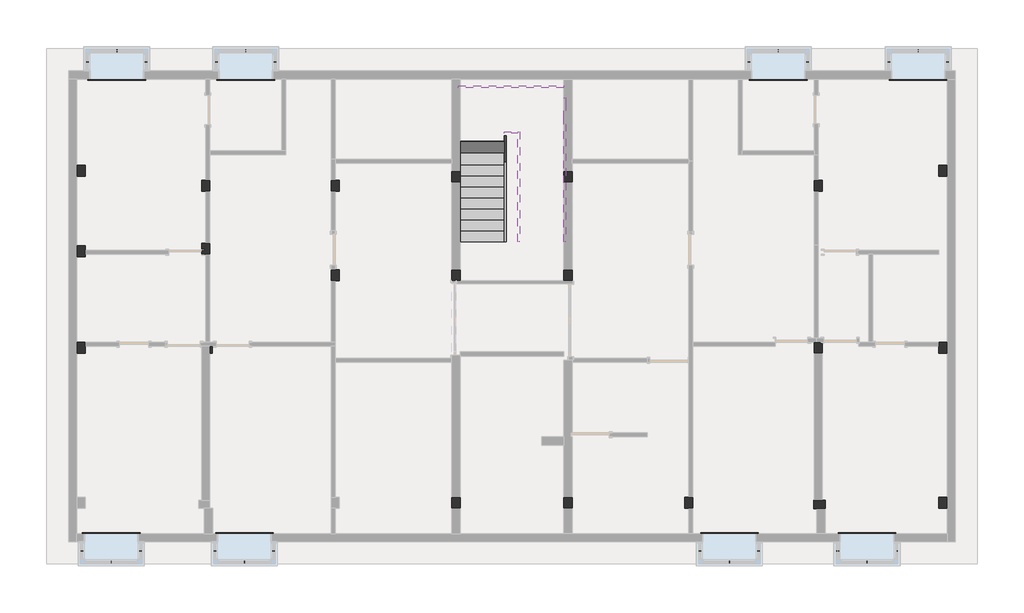
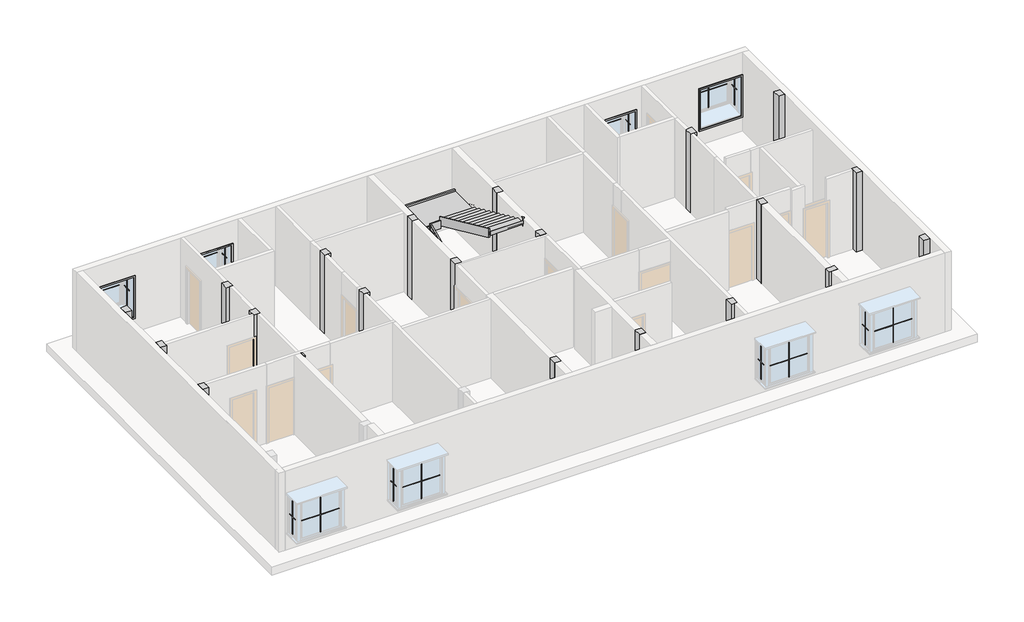
# One storey, part 3 of 3: 32 proxies, 21 columns, 6 members, 1 stair flight.
"""IFC4 building model written with IfcOpenShell, lengths in millimetres."""

from ifc_helpers import new_model, si_unit, frame, origin, place, context, project, spatial, polyline, outline, extrude, faceted_brep, transform, mapped, element, save
from components import m_muntin_pattern_2x2_m_muntin_pattern_2x2_c1fd4460, m_muntin_pattern_2x2_m_muntin_pattern_2x2_777b163a, m_trim_window_interior_flat_picture_frame_44e8afef, stair_flight_5ae6432b

model = new_model("IFC4")

# Units and contexts
model_context = context("Model", 3, world=origin())
ifc_project = project(units=[si_unit("LENGTHUNIT", "METRE", prefix="MILLI")], contexts=[model_context])

# Site, building, storey
site = spatial("IfcSite", under=ifc_project)
building = spatial("IfcBuilding", under=site)
storey = spatial("IfcBuildingStorey", under=building, Elevation=6400.8)

# Proxies
placement = place(None, origin())
m_muntin_pattern_2x2_m_muntin_pattern_2x2_shape = m_muntin_pattern_2x2_m_muntin_pattern_2x2_c1fd4460(model_context)
element("IfcBuildingElementProxy", 1, Name="M_Muntin Pattern_2x2 : M_Muntin Pattern_2x2", ObjectType="M_Muntin Pattern_2x2 : M_Muntin Pattern_2x2", at=placement, inside=storey, context=model_context, shape_type="MappedRepresentation", body=[
    mapped(m_muntin_pattern_2x2_m_muntin_pattern_2x2_shape, transform((-11500.7987957, -5499.9182661, 7121.45), x_axis=(-1.0, 0.0, 0.0), y_axis=(0.0, -1.0, 0.0), z_axis=(0.0, 0.0, 1.0))),
])
element("IfcBuildingElementProxy", 2, Name="M_Muntin Pattern_2x2 : M_Muntin Pattern_2x2", ObjectType="M_Muntin Pattern_2x2 : M_Muntin Pattern_2x2", at=placement, inside=storey, context=model_context, shape_type="MappedRepresentation", body=[
    mapped(m_muntin_pattern_2x2_m_muntin_pattern_2x2_shape, transform((-7819.250543, -5499.9182661, 7121.45), x_axis=(-1.0, 0.0, 0.0), y_axis=(0.0, -1.0, 0.0), z_axis=(0.0, 0.0, 1.0))),
])
element("IfcBuildingElementProxy", 3, Name="M_Muntin Pattern_2x2 : M_Muntin Pattern_2x2", ObjectType="M_Muntin Pattern_2x2 : M_Muntin Pattern_2x2", at=placement, inside=storey, context=model_context, shape_type="MappedRepresentation", body=[
    mapped(m_muntin_pattern_2x2_m_muntin_pattern_2x2_shape, transform((5599.7512082, -5499.9182661, 7121.45), x_axis=(-1.0, 0.0, 0.0), y_axis=(0.0, -1.0, 0.0), z_axis=(0.0, 0.0, 1.0))),
])
element("IfcBuildingElementProxy", 4, Name="M_Muntin Pattern_2x2 : M_Muntin Pattern_2x2", ObjectType="M_Muntin Pattern_2x2 : M_Muntin Pattern_2x2", at=placement, inside=storey, context=model_context, shape_type="MappedRepresentation", body=[
    mapped(m_muntin_pattern_2x2_m_muntin_pattern_2x2_shape, transform((9408.6146942, -5499.9182662, 7121.45), x_axis=(-1.0, 0.0, 0.0), y_axis=(0.0, -1.0, 0.0), z_axis=(0.0, 0.0, 1.0))),
])
element("IfcBuildingElementProxy", 5, Name="M_Muntin Pattern_2x2 : M_Muntin Pattern_2x2", ObjectType="M_Muntin Pattern_2x2 : M_Muntin Pattern_2x2", at=placement, inside=storey, context=model_context, shape_type="MappedRepresentation", body=[
    mapped(m_muntin_pattern_2x2_m_muntin_pattern_2x2_shape, transform((-11348.3987957, 8647.7317329, 7121.45), x_axis=(1.0, 0.0, 0.0), y_axis=(0.0, 1.0, 0.0), z_axis=(0.0, 0.0, 1.0))),
])
element("IfcBuildingElementProxy", 6, Name="M_Muntin Pattern_2x2 : M_Muntin Pattern_2x2", ObjectType="M_Muntin Pattern_2x2 : M_Muntin Pattern_2x2", at=placement, inside=storey, context=model_context, shape_type="MappedRepresentation", body=[
    mapped(m_muntin_pattern_2x2_m_muntin_pattern_2x2_shape, transform((-7779.6987993, 8647.7317329, 7121.45), x_axis=(1.0, 0.0, 0.0), y_axis=(0.0, 1.0, 0.0), z_axis=(0.0, 0.0, 1.0))),
])
element("IfcBuildingElementProxy", 7, Name="M_Muntin Pattern_2x2 : M_Muntin Pattern_2x2", ObjectType="M_Muntin Pattern_2x2 : M_Muntin Pattern_2x2", at=placement, inside=storey, context=model_context, shape_type="MappedRepresentation", body=[
    mapped(m_muntin_pattern_2x2_m_muntin_pattern_2x2_shape, transform((6952.301208, 8647.7317329, 7121.45), x_axis=(1.0, 0.0, 0.0), y_axis=(0.0, 1.0, 0.0), z_axis=(0.0, 0.0, 1.0))),
])
element("IfcBuildingElementProxy", 8, Name="M_Muntin Pattern_2x2 : M_Muntin Pattern_2x2", ObjectType="M_Muntin Pattern_2x2 : M_Muntin Pattern_2x2", at=placement, inside=storey, context=model_context, shape_type="MappedRepresentation", body=[
    mapped(m_muntin_pattern_2x2_m_muntin_pattern_2x2_shape, transform((10825.8012075, 8647.7317329, 7121.45), x_axis=(1.0, 0.0, 0.0), y_axis=(0.0, 1.0, 0.0), z_axis=(0.0, 0.0, 1.0))),
])
m_muntin_pattern_2x2_m_muntin_pattern_2x2_2_shape = m_muntin_pattern_2x2_m_muntin_pattern_2x2_777b163a(model_context)
element("IfcBuildingElementProxy", 9, Name="M_Muntin Pattern_2x2 : M_Muntin Pattern_2x2", ObjectType="M_Muntin Pattern_2x2 : M_Muntin Pattern_2x2", at=placement, inside=storey, context=model_context, shape_type="MappedRepresentation", body=[
    mapped(m_muntin_pattern_2x2_m_muntin_pattern_2x2_2_shape, transform((-10690.4737957, -5190.3932661, 7121.45), x_axis=(0.0, 1.0, 0.0), y_axis=(-1.0, 0.0, 0.0), z_axis=(0.0, 0.0, 1.0))),
])
element("IfcBuildingElementProxy", 10, Name="M_Muntin Pattern_2x2 : M_Muntin Pattern_2x2", ObjectType="M_Muntin Pattern_2x2 : M_Muntin Pattern_2x2", at=placement, inside=storey, context=model_context, shape_type="MappedRepresentation", body=[
    mapped(m_muntin_pattern_2x2_m_muntin_pattern_2x2_2_shape, transform((-12311.1237957, -5190.3932661, 7121.45), x_axis=(0.0, -1.0, 0.0), y_axis=(1.0, 0.0, 0.0), z_axis=(0.0, 0.0, 1.0))),
])
element("IfcBuildingElementProxy", 11, Name="M_Muntin Pattern_2x2 : M_Muntin Pattern_2x2", ObjectType="M_Muntin Pattern_2x2 : M_Muntin Pattern_2x2", at=placement, inside=storey, context=model_context, shape_type="MappedRepresentation", body=[
    mapped(m_muntin_pattern_2x2_m_muntin_pattern_2x2_2_shape, transform((-7008.925543, -5190.3932661, 7121.45), x_axis=(0.0, 1.0, 0.0), y_axis=(-1.0, 0.0, 0.0), z_axis=(0.0, 0.0, 1.0))),
])
element("IfcBuildingElementProxy", 12, Name="M_Muntin Pattern_2x2 : M_Muntin Pattern_2x2", ObjectType="M_Muntin Pattern_2x2 : M_Muntin Pattern_2x2", at=placement, inside=storey, context=model_context, shape_type="MappedRepresentation", body=[
    mapped(m_muntin_pattern_2x2_m_muntin_pattern_2x2_2_shape, transform((-8629.575543, -5190.3932661, 7121.45), x_axis=(0.0, -1.0, 0.0), y_axis=(1.0, 0.0, 0.0), z_axis=(0.0, 0.0, 1.0))),
])
element("IfcBuildingElementProxy", 13, Name="M_Muntin Pattern_2x2 : M_Muntin Pattern_2x2", ObjectType="M_Muntin Pattern_2x2 : M_Muntin Pattern_2x2", at=placement, inside=storey, context=model_context, shape_type="MappedRepresentation", body=[
    mapped(m_muntin_pattern_2x2_m_muntin_pattern_2x2_2_shape, transform((6410.0762082, -5190.3932661, 7121.45), x_axis=(0.0, 1.0, 0.0), y_axis=(-1.0, 0.0, 0.0), z_axis=(0.0, 0.0, 1.0))),
])
element("IfcBuildingElementProxy", 14, Name="M_Muntin Pattern_2x2 : M_Muntin Pattern_2x2", ObjectType="M_Muntin Pattern_2x2 : M_Muntin Pattern_2x2", at=placement, inside=storey, context=model_context, shape_type="MappedRepresentation", body=[
    mapped(m_muntin_pattern_2x2_m_muntin_pattern_2x2_2_shape, transform((4789.4262082, -5190.3932661, 7121.45), x_axis=(0.0, -1.0, 0.0), y_axis=(1.0, 0.0, 0.0), z_axis=(0.0, 0.0, 1.0))),
])
element("IfcBuildingElementProxy", 15, Name="M_Muntin Pattern_2x2 : M_Muntin Pattern_2x2", ObjectType="M_Muntin Pattern_2x2 : M_Muntin Pattern_2x2", at=placement, inside=storey, context=model_context, shape_type="MappedRepresentation", body=[
    mapped(m_muntin_pattern_2x2_m_muntin_pattern_2x2_2_shape, transform((10218.9396942, -5190.3932662, 7121.45), x_axis=(0.0, 1.0, 0.0), y_axis=(-1.0, 0.0, 0.0), z_axis=(0.0, 0.0, 1.0))),
])
element("IfcBuildingElementProxy", 16, Name="M_Muntin Pattern_2x2 : M_Muntin Pattern_2x2", ObjectType="M_Muntin Pattern_2x2 : M_Muntin Pattern_2x2", at=placement, inside=storey, context=model_context, shape_type="MappedRepresentation", body=[
    mapped(m_muntin_pattern_2x2_m_muntin_pattern_2x2_2_shape, transform((8598.2896942, -5190.3932661, 7121.45), x_axis=(0.0, -1.0, 0.0), y_axis=(1.0, 0.0, 0.0), z_axis=(0.0, 0.0, 1.0))),
])
element("IfcBuildingElementProxy", 17, Name="M_Muntin Pattern_2x2 : M_Muntin Pattern_2x2", ObjectType="M_Muntin Pattern_2x2 : M_Muntin Pattern_2x2", at=placement, inside=storey, context=model_context, shape_type="MappedRepresentation", body=[
    mapped(m_muntin_pattern_2x2_m_muntin_pattern_2x2_2_shape, transform((-12158.7237957, 8338.2067329, 7121.45), x_axis=(0.0, -1.0, 0.0), y_axis=(1.0, 0.0, 0.0), z_axis=(0.0, 0.0, 1.0))),
])
element("IfcBuildingElementProxy", 18, Name="M_Muntin Pattern_2x2 : M_Muntin Pattern_2x2", ObjectType="M_Muntin Pattern_2x2 : M_Muntin Pattern_2x2", at=placement, inside=storey, context=model_context, shape_type="MappedRepresentation", body=[
    mapped(m_muntin_pattern_2x2_m_muntin_pattern_2x2_2_shape, transform((-10538.0737957, 8338.2067329, 7121.45), x_axis=(0.0, 1.0, 0.0), y_axis=(-1.0, 0.0, 0.0), z_axis=(0.0, 0.0, 1.0))),
])
element("IfcBuildingElementProxy", 19, Name="M_Muntin Pattern_2x2 : M_Muntin Pattern_2x2", ObjectType="M_Muntin Pattern_2x2 : M_Muntin Pattern_2x2", at=placement, inside=storey, context=model_context, shape_type="MappedRepresentation", body=[
    mapped(m_muntin_pattern_2x2_m_muntin_pattern_2x2_2_shape, transform((-8590.0237993, 8338.2067329, 7121.45), x_axis=(0.0, -1.0, 0.0), y_axis=(1.0, 0.0, 0.0), z_axis=(0.0, 0.0, 1.0))),
])
element("IfcBuildingElementProxy", 20, Name="M_Muntin Pattern_2x2 : M_Muntin Pattern_2x2", ObjectType="M_Muntin Pattern_2x2 : M_Muntin Pattern_2x2", at=placement, inside=storey, context=model_context, shape_type="MappedRepresentation", body=[
    mapped(m_muntin_pattern_2x2_m_muntin_pattern_2x2_2_shape, transform((-6969.3737993, 8338.2067329, 7121.45), x_axis=(0.0, 1.0, 0.0), y_axis=(-1.0, 0.0, 0.0), z_axis=(0.0, 0.0, 1.0))),
])
element("IfcBuildingElementProxy", 21, Name="M_Muntin Pattern_2x2 : M_Muntin Pattern_2x2", ObjectType="M_Muntin Pattern_2x2 : M_Muntin Pattern_2x2", at=placement, inside=storey, context=model_context, shape_type="MappedRepresentation", body=[
    mapped(m_muntin_pattern_2x2_m_muntin_pattern_2x2_2_shape, transform((6141.976208, 8338.2067329, 7121.45), x_axis=(0.0, -1.0, 0.0), y_axis=(1.0, 0.0, 0.0), z_axis=(0.0, 0.0, 1.0))),
])
element("IfcBuildingElementProxy", 22, Name="M_Muntin Pattern_2x2 : M_Muntin Pattern_2x2", ObjectType="M_Muntin Pattern_2x2 : M_Muntin Pattern_2x2", at=placement, inside=storey, context=model_context, shape_type="MappedRepresentation", body=[
    mapped(m_muntin_pattern_2x2_m_muntin_pattern_2x2_2_shape, transform((7762.626208, 8338.2067329, 7121.45), x_axis=(0.0, 1.0, 0.0), y_axis=(-1.0, 0.0, 0.0), z_axis=(0.0, 0.0, 1.0))),
])
element("IfcBuildingElementProxy", 23, Name="M_Muntin Pattern_2x2 : M_Muntin Pattern_2x2", ObjectType="M_Muntin Pattern_2x2 : M_Muntin Pattern_2x2", at=placement, inside=storey, context=model_context, shape_type="MappedRepresentation", body=[
    mapped(m_muntin_pattern_2x2_m_muntin_pattern_2x2_2_shape, transform((10015.4762075, 8338.2067329, 7121.45), x_axis=(0.0, -1.0, 0.0), y_axis=(1.0, 0.0, 0.0), z_axis=(0.0, 0.0, 1.0))),
])
element("IfcBuildingElementProxy", 24, Name="M_Muntin Pattern_2x2 : M_Muntin Pattern_2x2", ObjectType="M_Muntin Pattern_2x2 : M_Muntin Pattern_2x2", at=placement, inside=storey, context=model_context, shape_type="MappedRepresentation", body=[
    mapped(m_muntin_pattern_2x2_m_muntin_pattern_2x2_2_shape, transform((11636.1262075, 8338.2067329, 7121.45), x_axis=(0.0, 1.0, 0.0), y_axis=(-1.0, 0.0, 0.0), z_axis=(0.0, 0.0, 1.0))),
])
m_trim_window_interior_flat_picture_frame_shape = m_trim_window_interior_flat_picture_frame_44e8afef(model_context)
element("IfcBuildingElementProxy", 25, Name="M_Trim-Window-Interior-Flat : Picture Frame", ObjectType="M_Trim-Window-Interior-Flat : Picture Frame", at=placement, inside=storey, context=model_context, shape_type="MappedRepresentation", body=[
    mapped(m_trim_window_interior_flat_picture_frame_shape, transform((-11500.7987957, -4712.5932661, 8551.6), x_axis=(-1.0, 0.0, 0.0), y_axis=(0.0, 0.0, 1.0), z_axis=(0.0, 1.0, 0.0))),
])
element("IfcBuildingElementProxy", 26, Name="M_Trim-Window-Interior-Flat : Picture Frame", ObjectType="M_Trim-Window-Interior-Flat : Picture Frame", at=placement, inside=storey, context=model_context, shape_type="MappedRepresentation", body=[
    mapped(m_trim_window_interior_flat_picture_frame_shape, transform((-7819.250543, -4712.5932661, 8551.6), x_axis=(-1.0, 0.0, 0.0), y_axis=(0.0, 0.0, 1.0), z_axis=(0.0, 1.0, 0.0))),
])
element("IfcBuildingElementProxy", 27, Name="M_Trim-Window-Interior-Flat : Picture Frame", ObjectType="M_Trim-Window-Interior-Flat : Picture Frame", at=placement, inside=storey, context=model_context, shape_type="MappedRepresentation", body=[
    mapped(m_trim_window_interior_flat_picture_frame_shape, transform((5599.7512082, -4712.5932661, 8551.6), x_axis=(-1.0, 0.0, 0.0), y_axis=(0.0, 0.0, 1.0), z_axis=(0.0, 1.0, 0.0))),
])
element("IfcBuildingElementProxy", 28, Name="M_Trim-Window-Interior-Flat : Picture Frame", ObjectType="M_Trim-Window-Interior-Flat : Picture Frame", at=placement, inside=storey, context=model_context, shape_type="MappedRepresentation", body=[
    mapped(m_trim_window_interior_flat_picture_frame_shape, transform((9408.6146942, -4712.5932661, 8551.6), x_axis=(-1.0, 0.0, 0.0), y_axis=(0.0, 0.0, 1.0), z_axis=(0.0, 1.0, 0.0))),
])
element("IfcBuildingElementProxy", 29, Name="M_Trim-Window-Interior-Flat : Picture Frame", ObjectType="M_Trim-Window-Interior-Flat : Picture Frame", at=placement, inside=storey, context=model_context, shape_type="MappedRepresentation", body=[
    mapped(m_trim_window_interior_flat_picture_frame_shape, transform((-11348.3987957, 7860.4067329, 8551.6), x_axis=(1.0, 0.0, 0.0), y_axis=(0.0, 0.0, 1.0), z_axis=(0.0, -1.0, 0.0))),
])
element("IfcBuildingElementProxy", 30, Name="M_Trim-Window-Interior-Flat : Picture Frame", ObjectType="M_Trim-Window-Interior-Flat : Picture Frame", at=placement, inside=storey, context=model_context, shape_type="MappedRepresentation", body=[
    mapped(m_trim_window_interior_flat_picture_frame_shape, transform((-7779.6987993, 7860.4067329, 8551.6), x_axis=(1.0, 0.0, 0.0), y_axis=(0.0, 0.0, 1.0), z_axis=(0.0, -1.0, 0.0))),
])
element("IfcBuildingElementProxy", 31, Name="M_Trim-Window-Interior-Flat : Picture Frame", ObjectType="M_Trim-Window-Interior-Flat : Picture Frame", at=placement, inside=storey, context=model_context, shape_type="MappedRepresentation", body=[
    mapped(m_trim_window_interior_flat_picture_frame_shape, transform((6952.301208, 7860.4067329, 8551.6), x_axis=(1.0, 0.0, 0.0), y_axis=(0.0, 0.0, 1.0), z_axis=(0.0, -1.0, 0.0))),
])
element("IfcBuildingElementProxy", 32, Name="M_Trim-Window-Interior-Flat : Picture Frame", ObjectType="M_Trim-Window-Interior-Flat : Picture Frame", at=placement, inside=storey, context=model_context, shape_type="MappedRepresentation", body=[
    mapped(m_trim_window_interior_flat_picture_frame_shape, transform((10825.8012075, 7860.4067329, 8551.6), x_axis=(1.0, 0.0, 0.0), y_axis=(0.0, 0.0, 1.0), z_axis=(0.0, -1.0, 0.0))),
])

# Columns
element("IfcColumn", 33, ObjectType="Rectangular Column : 1'X 9\"", at=placement, inside=storey, context=model_context, shape_type="SweptSolid", body=[
    extrude(outline(polyline([(-12224.6987957, 583.3067334), (-12224.6987957, 278.5067334), (-12453.2987957, 278.5067334), (-12453.2987957, 583.3067334), (-12224.6987957, 583.3067334)])), frame((0.0, 0.0, 6400.8), z_axis=(0.0, 0.0, 1.0), x_axis=(1.0, 0.0, 0.0)), (0.0, 0.0, 1.0), 3048.0),
])
element("IfcColumn", 34, ObjectType="Rectangular Column : 1'X 9\"", at=placement, inside=storey, context=model_context, shape_type="SweptSolid", body=[
    extrude(outline(polyline([(-12224.6987957, 3256.6567332), (-12224.6987957, 2951.8567332), (-12453.2987957, 2951.8567332), (-12453.2987957, 3256.6567332), (-12224.6987957, 3256.6567332)])), frame((0.0, 0.0, 6400.8), z_axis=(0.0, 0.0, 1.0), x_axis=(1.0, 0.0, 0.0)), (0.0, 0.0, 1.0), 3048.0),
])
element("IfcColumn", 35, ObjectType="Rectangular Column : 1'X 9\"", at=placement, inside=storey, context=model_context, shape_type="Brep", body=[
    faceted_brep([(-8770.2987992, 5066.406733, 6400.8), (-8770.2987992, 4761.606733, 6400.8), (-8884.5987992, 4761.606733, 6400.8), (-8998.8987992, 4761.606733, 6400.8), (-8998.8987992, 5066.406733, 6400.8), (-8884.5987992, 5066.406733, 6400.8), (-8770.2987992, 5066.406733, 9448.8), (-8770.2987992, 4761.606733, 9448.8), (-8884.5987992, 4761.606733, 9448.8), (-8998.8987992, 4761.606733, 9448.8), (-8998.8987992, 5066.406733, 9448.8), (-8884.5987992, 5066.406733, 9448.8)], [[[0, 1, 2, 3, 4, 5]], [[6, 7, 1, 0]], [[7, 8, 9, 3, 2, 1]], [[9, 10, 4, 3]], [[10, 11, 6, 0, 5, 4]], [[6, 11, 10, 9, 8, 7]]]),
])
element("IfcColumn", 36, ObjectType="Rectangular Column : 1'X 9\"", at=placement, inside=storey, context=model_context, shape_type="Brep", body=[
    faceted_brep([(-8770.2987992, 3326.5067332, 6400.8), (-8770.2987992, 3021.7067332, 6400.8), (-8884.598796, 3021.7067332, 6400.8), (-8998.8987992, 3021.7067332, 6400.8), (-8998.8987992, 3326.5067332, 6400.8), (-8884.5987992, 3326.5067332, 6400.8), (-8770.2987992, 3326.5067332, 9448.8), (-8770.2987992, 3021.7067332, 9448.8), (-8884.598796, 3021.7067332, 9448.8), (-8998.8987992, 3021.7067332, 9448.8), (-8998.8987992, 3326.5067332, 9448.8), (-8884.5987992, 3326.5067332, 9448.8)], [[[0, 1, 2, 3, 4, 5]], [[6, 7, 1, 0]], [[7, 8, 9, 3, 2, 1]], [[9, 10, 4, 3]], [[10, 11, 6, 0, 5, 4]], [[6, 11, 10, 9, 8, 7]]]),
])
element("IfcColumn", 37, ObjectType="Rectangular Column : 1'X 9\"", at=placement, inside=storey, context=model_context, shape_type="SweptSolid", body=[
    extrude(outline(polyline([(-8713.148796, 278.5067334), (-8771.750543, 278.5067334), (-8771.750543, 469.0067334), (-8713.148796, 469.0067334), (-8713.148796, 278.5067334)])), frame((0.0, 0.0, 6400.8), z_axis=(0.0, 0.0, 1.0), x_axis=(1.0, 0.0, 0.0)), (0.0, 0.0, 1.0), 3048.0),
])
element("IfcColumn", 38, ObjectType="Rectangular Column : 1'X 9\"", at=placement, inside=storey, context=model_context, shape_type="Brep", body=[
    faceted_brep([(-5188.8987995, 5066.406733, 6400.8), (-5188.8987995, 4761.606733, 6400.8), (-5303.1987995, 4761.606733, 6400.8), (-5417.4987995, 4761.606733, 6400.8), (-5417.4987995, 5066.406733, 6400.8), (-5303.1987995, 5066.406733, 6400.8), (-5188.8987995, 5066.406733, 9448.8), (-5188.8987995, 4761.606733, 9448.8), (-5303.1987995, 4761.606733, 9448.8), (-5417.4987995, 4761.606733, 9448.8), (-5417.4987995, 5066.406733, 9448.8), (-5303.1987995, 5066.406733, 9448.8)], [[[0, 1, 2, 3, 4, 5]], [[6, 7, 1, 0]], [[7, 8, 9, 3, 2, 1]], [[9, 10, 4, 3]], [[10, 11, 6, 0, 5, 4]], [[6, 11, 10, 9, 8, 7]]]),
])
element("IfcColumn", 39, ObjectType="Rectangular Column : 1'X 9\"", at=placement, inside=storey, context=model_context, shape_type="Brep", body=[
    faceted_brep([(-5188.8987995, 2589.9067802, 6400.8), (-5188.8987995, 2285.1067802, 6400.8), (-5303.1987995, 2285.1067802, 6400.8), (-5417.4987995, 2285.1067802, 6400.8), (-5417.4987995, 2589.9067802, 6400.8), (-5303.1987995, 2589.9067802, 6400.8), (-5188.8987995, 2589.9067802, 9448.8), (-5188.8987995, 2285.1067802, 9448.8), (-5303.1987995, 2285.1067802, 9448.8), (-5417.4987995, 2285.1067802, 9448.8), (-5417.4987995, 2589.9067802, 9448.8), (-5303.1987995, 2589.9067802, 9448.8)], [[[0, 1, 2, 3, 4, 5]], [[6, 7, 1, 0]], [[7, 8, 9, 3, 2, 1]], [[9, 10, 4, 3]], [[10, 11, 6, 0, 5, 4]], [[6, 11, 10, 9, 8, 7]]]),
])
element("IfcColumn", 40, ObjectType="Rectangular Column : 1'X 9\"", at=placement, inside=storey, context=model_context, shape_type="SweptSolid", body=[
    extrude(outline(polyline([(1250.0012085, -3709.2932193), (1250.0012085, -4014.0932193), (1021.4012085, -4014.0932193), (1021.4012085, -3709.2932193), (1250.0012085, -3709.2932193)])), frame((0.0, 0.0, 6400.8), z_axis=(0.0, 0.0, 1.0), x_axis=(1.0, 0.0, 0.0)), (0.0, 0.0, 1.0), 3048.0),
])
element("IfcColumn", 41, ObjectType="Rectangular Column : 1'X 9\"", at=placement, inside=storey, context=model_context, shape_type="Brep", body=[
    faceted_brep([(4590.1012082, -3709.2932193, 6400.8), (4590.1012082, -4014.0932193, 6400.8), (4475.8012082, -4014.0932193, 6400.8), (4361.5012082, -4014.0932193, 6400.8), (4361.5012082, -3709.2932193, 6400.8), (4475.8012082, -3709.2932193, 6400.8), (4590.1012082, -3709.2932193, 9448.8), (4590.1012082, -4014.0932193, 9448.8), (4475.8012082, -4014.0932193, 9448.8), (4361.5012082, -4014.0932193, 9448.8), (4361.5012082, -3709.2932193, 9448.8), (4475.8012082, -3709.2932193, 9448.8)], [[[0, 1, 2, 3, 4, 5]], [[6, 7, 1, 0]], [[7, 8, 9, 3, 2, 1]], [[9, 10, 4, 3]], [[10, 11, 6, 0, 5, 4]], [[6, 11, 10, 9, 8, 7]]]),
])
element("IfcColumn", 42, ObjectType="Rectangular Column : 1'X 9\"", at=placement, inside=storey, context=model_context, shape_type="SweptSolid", body=[
    extrude(outline(polyline([(11625.9012075, -3709.2932671), (11625.9012075, -4014.0932671), (11397.3012075, -4014.0932671), (11397.3012075, -3709.2932671), (11625.9012075, -3709.2932671)])), frame((0.0, 0.0, 6400.8), z_axis=(0.0, 0.0, 1.0), x_axis=(1.0, 0.0, 0.0)), (0.0, 0.0, 1.0), 3048.0),
])
element("IfcColumn", 43, ObjectType="Rectangular Column : 1'X 9\"", at=placement, inside=storey, context=model_context, shape_type="Brep", body=[
    faceted_brep([(11625.9012075, 583.3067295, 6400.8), (11625.9012075, 278.5067295, 6400.8), (11397.3012075, 278.5067295, 6400.8), (11397.3012075, 469.0067295, 6400.8), (11397.3012075, 583.3067295, 6400.8), (11625.9012075, 583.3067295, 9448.8), (11625.9012075, 278.5067295, 9448.8), (11397.3012075, 278.5067295, 9448.8), (11397.3012075, 469.0067295, 9448.8), (11397.3012075, 583.3067295, 9448.8)], [[[0, 1, 2, 3, 4]], [[5, 6, 1, 0]], [[6, 7, 2, 1]], [[7, 8, 9, 4, 3, 2]], [[9, 5, 0, 4]], [[5, 9, 8, 7, 6]]]),
])
element("IfcColumn", 44, ObjectType="Rectangular Column : 1'X 9\"", at=placement, inside=storey, context=model_context, shape_type="SweptSolid", body=[
    extrude(outline(polyline([(11625.9012075, 5479.1567329), (11625.9012075, 5174.3567329), (11397.3012075, 5174.3567329), (11397.3012075, 5479.1567329), (11625.9012075, 5479.1567329)])), frame((0.0, 0.0, 6400.8), z_axis=(0.0, 0.0, 1.0), x_axis=(1.0, 0.0, 0.0)), (0.0, 0.0, 1.0), 3048.0),
])
element("IfcColumn", 45, ObjectType="Rectangular Column : 1'X 9\"", at=placement, inside=storey, context=model_context, shape_type="Brep", body=[
    faceted_brep([(8172.5040565, 5065.4824989, 6400.8), (8172.5040565, 4760.6824989, 6400.8), (8057.2012047, 4760.6824989, 6400.8), (7943.9040565, 4760.6824989, 6400.8), (7943.9040565, 5065.4824989, 6400.8), (8058.2040565, 5065.4824989, 6400.8), (8172.5040565, 5065.4824989, 9448.8), (8172.5040565, 4760.6824989, 9448.8), (8057.2012047, 4760.6824989, 9448.8), (7943.9040565, 4760.6824989, 9448.8), (7943.9040565, 5065.4824989, 9448.8), (8058.2040565, 5065.4824989, 9448.8)], [[[0, 1, 2, 3, 4, 5]], [[6, 7, 1, 0]], [[7, 8, 9, 3, 2, 1]], [[9, 10, 4, 3]], [[10, 11, 6, 0, 5, 4]], [[6, 11, 10, 9, 8, 7]]]),
])
element("IfcColumn", 46, ObjectType="Rectangular Column : 1'X 9\"", at=placement, inside=storey, context=model_context, shape_type="Brep", body=[
    faceted_brep([(8171.5012047, 583.3067334, 6400.8), (8171.5012047, 278.5067334, 6400.8), (7942.9012047, 278.5067334, 6400.8), (7942.9012047, 583.3067334, 6400.8), (8000.0512079, 583.3067334, 6400.8), (8171.5012047, 583.3067334, 9448.8), (8171.5012047, 278.5067334, 9448.8), (7942.9012047, 278.5067334, 9448.8), (7942.9012047, 583.3067334, 9448.8), (8000.0512079, 583.3067334, 9448.8)], [[[0, 1, 2, 3, 4]], [[5, 6, 1, 0]], [[6, 7, 2, 1]], [[7, 8, 3, 2]], [[8, 9, 5, 0, 4, 3]], [[5, 9, 8, 7, 6]]]),
])
element("IfcColumn", 47, ObjectType="Rectangular Column : 1'X 9\"", at=placement, inside=storey, context=model_context, shape_type="Brep", body=[
    faceted_brep([(7941.7646942, -3787.3914801, 6400.8), (8246.5646942, -3787.3914801, 6400.8), (8246.5646942, -4015.9914801, 6400.8), (8017.9646942, -4015.9914801, 6400.8), (7941.7646942, -4015.9914801, 6400.8), (7941.7646942, -3787.3914801, 9448.8), (8246.5646942, -3787.3914801, 9448.8), (8246.5646942, -4015.9914801, 9448.8), (8017.9646942, -4015.9914801, 9448.8), (7941.7646942, -4015.9914801, 9448.8)], [[[0, 1, 2, 3, 4]], [[5, 6, 1, 0]], [[6, 7, 2, 1]], [[7, 8, 9, 4, 3, 2]], [[9, 5, 0, 4]], [[5, 9, 8, 7, 6]]]),
])
element("IfcColumn", 48, ObjectType="Rectangular Column : 1'X 9\"", at=placement, inside=storey, context=model_context, shape_type="SweptSolid", body=[
    extrude(outline(polyline([(-12453.2987957, 5174.3567339), (-12453.2987957, 5479.1567339), (-12224.6987957, 5479.1567339), (-12224.6987957, 5174.3567339), (-12453.2987957, 5174.3567339)])), frame((0.0, 0.0, 6400.8), z_axis=(0.0, 0.0, 1.0), x_axis=(1.0, 0.0, 0.0)), (0.0, 0.0, 1.0), 3048.0),
])
element("IfcColumn", 49, ObjectType="Rectangular Column : 1'X 9\"", at=placement, inside=storey, context=model_context, shape_type="SweptSolid", body=[
    extrude(outline(polyline([(-1845.5417538, 5320.4067329), (-1845.5417538, 5015.6067329), (-2074.1417538, 5015.6067329), (-2074.1417538, 5320.4067329), (-1845.5417538, 5320.4067329)])), frame((0.0, 0.0, 6400.8), z_axis=(0.0, 0.0, 1.0), x_axis=(1.0, 0.0, 0.0)), (0.0, 0.0, 1.0), 3048.0),
])
element("IfcColumn", 50, ObjectType="Rectangular Column : 1'X 9\"", at=placement, inside=storey, context=model_context, shape_type="SweptSolid", body=[
    extrude(outline(polyline([(1250.0012085, 5320.4067329), (1250.0012085, 5015.6067329), (1021.4012085, 5015.6067329), (1021.4012085, 5320.4067329), (1250.0012085, 5320.4067329)])), frame((0.0, 0.0, 6400.8), z_axis=(0.0, 0.0, 1.0), x_axis=(1.0, 0.0, 0.0)), (0.0, 0.0, 1.0), 3048.0),
])
element("IfcColumn", 51, ObjectType="Rectangular Column : 1'X 9\"", at=placement, inside=storey, context=model_context, shape_type="SweptSolid", body=[
    extrude(outline(polyline([(-1845.5417538, 2589.906774), (-1845.5417538, 2285.106774), (-2074.1417538, 2285.106774), (-2074.1417538, 2589.906774), (-1845.5417538, 2589.906774)])), frame((0.0, 0.0, 6400.8), z_axis=(0.0, 0.0, 1.0), x_axis=(1.0, 0.0, 0.0)), (0.0, 0.0, 1.0), 3048.0),
])
element("IfcColumn", 52, ObjectType="Rectangular Column : 1'X 9\"", at=placement, inside=storey, context=model_context, shape_type="Brep", body=[
    faceted_brep([(1253.2582462, 2589.9067742, 6400.8), (1253.2582462, 2285.1067742, 6400.8), (1024.6582462, 2285.1067742, 6400.8), (1024.6582462, 2589.9067742, 6400.8), (1250.0012085, 2589.9067742, 6400.8), (1253.2582462, 2589.9067742, 9448.8), (1253.2582462, 2285.1067742, 9448.8), (1024.6582462, 2285.1067742, 9448.8), (1024.6582462, 2589.9067742, 9448.8), (1250.0012085, 2589.9067742, 9448.8)], [[[0, 1, 2, 3, 4]], [[5, 6, 1, 0]], [[6, 7, 2, 1]], [[7, 8, 3, 2]], [[8, 9, 5, 0, 4, 3]], [[5, 9, 8, 7, 6]]]),
])
element("IfcColumn", 53, ObjectType="Rectangular Column : 1'X 9\"", at=placement, inside=storey, context=model_context, shape_type="SweptSolid", body=[
    extrude(outline(polyline([(-1848.7987998, -3709.2932663), (-1848.7987998, -4014.0932663), (-2077.3987998, -4014.0932663), (-2077.3987998, -3709.2932663), (-1848.7987998, -3709.2932663)])), frame((0.0, 0.0, 6400.8), z_axis=(0.0, 0.0, 1.0), x_axis=(1.0, 0.0, 0.0)), (0.0, 0.0, 1.0), 3048.0),
])

# Members
element("IfcMember", 54, ObjectType="Stringer - 2\" Width", at=placement, inside=storey, context=model_context, shape_type="SweptSolid", body=[
    extrude(outline(polyline([(3364.6067329, 6400.8), (3364.6067329, 6600.6262721), (6445.4289342, 8001.0), (7182.0114168, 8001.0), (3661.5714168, 6400.8), (3364.6067329, 6400.8)])), frame((-1896.3417538, 0.0, 0.0), z_axis=(1.0, 0.0, 0.0), x_axis=(0.0, 1.0, 0.0)), (0.0, 0.0, 1.0), 50.8),
])
element("IfcMember", 55, ObjectType="Stringer - 2\" Width", at=placement, inside=storey, context=model_context, shape_type="SweptSolid", body=[
    extrude(outline(polyline([(-1896.3417538, 7631.8067329), (-1896.3417538, 7682.6067329), (1021.4012085, 7682.6067329), (1021.4012085, 7631.8067329), (-1896.3417538, 7631.8067329)])), frame((0.0, 0.0, 7696.2), z_axis=(0.0, 0.0, 1.0), x_axis=(1.0, 0.0, 0.0)), (0.0, 0.0, 1.0), 304.8),
])
element("IfcMember", 56, ObjectType="Stringer - 2\" Width", at=placement, inside=storey, context=model_context, shape_type="SweptSolid", body=[
    extrude(outline(polyline([(6618.562049, 7696.2), (3364.6067329, 9175.2705982), (3364.6067329, 9510.0808176), (7355.1445316, 7696.2), (6618.562049, 7696.2)])), frame((1021.4012085, 0.0, 0.0), z_axis=(1.0, 0.0, 0.0), x_axis=(0.0, 1.0, 0.0)), (0.0, 0.0, 1.0), 50.8),
])
element("IfcMember", 57, ObjectType="Stringer - 2\" Width", at=placement, inside=storey, context=model_context, shape_type="SweptSolid", body=[
    extrude(outline(polyline([(3364.6067329, 6400.8), (3364.6067329, 6600.6262721), (6361.8067329, 7962.9899085), (6361.8067329, 7628.1796892), (3661.5714168, 6400.8), (3364.6067329, 6400.8)])), frame((-629.5987998, 0.0, 0.0), z_axis=(1.0, 0.0, 0.0), x_axis=(0.0, 1.0, 0.0)), (0.0, 0.0, 1.0), 50.8),
])
element("IfcMember", 58, ObjectType="Stringer - 2\" Width", at=placement, inside=storey, context=model_context, shape_type="SweptSolid", body=[
    extrude(outline(polyline([(-629.5987998, 6361.8067329), (-629.5987998, 6412.6067329), (-248.5987915, 6412.6067329), (-248.5987915, 6361.8067329), (-629.5987998, 6361.8067329)])), frame((0.0, 0.0, 7696.2), z_axis=(0.0, 0.0, 1.0), x_axis=(1.0, 0.0, 0.0)), (0.0, 0.0, 1.0), 304.8),
])
element("IfcMember", 59, ObjectType="Stringer - 2\" Width", at=placement, inside=storey, context=model_context, shape_type="SweptSolid", body=[
    extrude(outline(polyline([(6412.6067329, 8124.6262721), (6412.6067329, 7789.8160528), (3364.6067329, 9175.2705982), (3364.6067329, 9510.0808176), (6412.6067329, 8124.6262721)])), frame((-248.5987915, 0.0, 0.0), z_axis=(1.0, 0.0, 0.0), x_axis=(0.0, 1.0, 0.0)), (0.0, 0.0, 1.0), 50.8),
])

# Stair flight
stair_flight_shape = stair_flight_5ae6432b(model_context)
element("IfcStairFlight", 60, ObjectType="2\" Tread 1\" Nosing 1/4\" Riser", at=placement, inside=storey, context=model_context, shape_type="MappedRepresentation", body=[
    mapped(stair_flight_shape, transform((0.0, 0.0, 0.0), x_axis=(1.0, 0.0, 0.0), y_axis=(0.0, 1.0, 0.0), z_axis=(0.0, 0.0, 1.0))),
])

save(model, "model.ifc")

# Revit data of these elements
# Type "M_Muntin Pattern_2x2 : M_Muntin Pattern_2x2"
#   Width [instance default] = 3' - 11.24409"
#   Thickness = 0' - 0 1/2"
#   Height [instance default] = 3' - 11.24409"
#   Distance = 0' - 0 3/4"
#   Interior Material [instance default] = none
#   Exterior Material [instance default] = none
#   Default Elevation = 0
# Type "M_Trim-Window-Interior-Flat : Picture Frame"
#   Trim Thickness_Picture Frame = 0' - 1.1811"
#   Trim Width = 0' - 2.3622"
#   Trim Thickness_with Sill = 0' - 0.7874"
#   Sill Thickness = 0' - 1.1811"
#   Opening Width [instance default] = 1' - 11.62205"
#   Opening Height [instance default] = 2' - 11.43307"
#   Default Elevation = 3' - 11.24409"
#   Sill = no
#   Picture Frame = yes
#   Trim Material [instance default] = none
# Type "Rectangular Column : 1'X 9\""
#   Assembly Code = "B1010200"
#   Depth = 1' - 0"
#   Offset Base = 0' - 0"
#   Offset Top = 0' - 0"
#   Width = 0' - 9"
#   Material = none
# Elements 1, 2, 3, 4, 5, 6, 7, 8 (IfcBuildingElementProxy, "M_Muntin Pattern_2x2 : M_Muntin Pattern_2x2")
#   Width = 4' - 5.55512"
#   Height = 4' - 5.55512"
#   Interior Material = Wood - Stained
#   Exterior Material = Clad - White
#   Phase Created = New Construction
#   Materials on its faces: "Clad - White", "Wood - Stained"
# Elements 9, 10, 11, 12, 13, 14, 15, 16, 17, 18, 19, 20, 21, 22, 23, 24 (IfcBuildingElementProxy, "M_Muntin Pattern_2x2 : M_Muntin Pattern_2x2")
#   Width = 1' - 2.12205"
#   Height = 4' - 5.55512"
#   Interior Material = Wood - Stained
#   Exterior Material = Clad - White
#   Phase Created = New Construction
#   Materials on its faces: "Clad - White", "Wood - Stained"
# Elements 25, 26, 27, 28, 29, 30, 31, 32 (IfcBuildingElementProxy, "M_Trim-Window-Interior-Flat : Picture Frame")
#   Opening Width = 4' - 11.05512"
#   Opening Height = 5' - 1.05512"
#   Trim Material = Wood - Stained
#   Phase Created = New Construction
#   Materials on its faces: "Wood - Stained"
# Elements 33, 34, 35, 36, 37, 38, 39, 40, 41, 42, 43, 44, 45, 46, 47, 48, 49, 50, 51, 52 (IfcColumn, "Rectangular Column : 1'X 9\"")
#   Phase Created = New Construction
#   Materials on its faces: "Default Wall"
# Element 53 (IfcColumn, "Rectangular Column : 1'X 9\"")
#   Phase Created = New Construction
# Elements 54, 55, 56, 57, 58, 59 (IfcMember, "Stringer - 2\" Width")
#   Phase Created = New Construction
# Element 60 (IfcStairFlight, "2\" Tread 1\" Nosing 1/4\" Riser")
#   Phase Created = New Construction
# Materials
#   "Clad - White": class "Wood", colour RGB 242 242 238, transparency 0, Cost = 0
#   "Wood - Stained": class "Wood", colour RGB 224 178 126, transparency 0, Cost = 0
#   "Default Wall": colour RGB 128 128 128, transparency 0, Cost = 0
